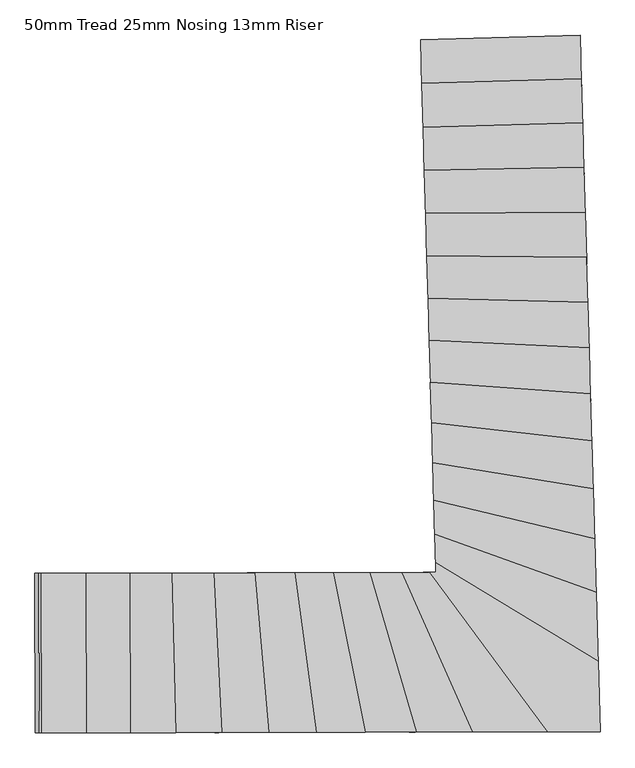
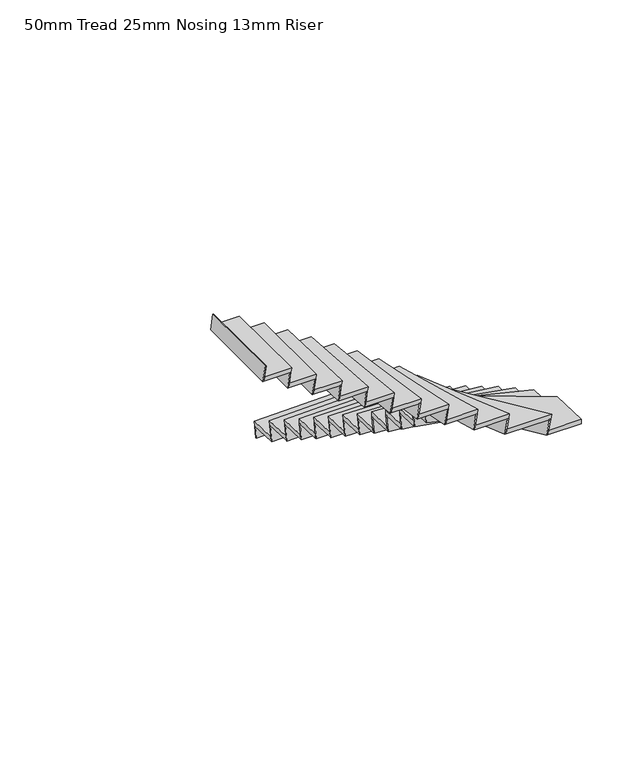
"""IFC4 building model written with IfcOpenShell, lengths in millimetres: stair flight geometry, 50mm Tread 25mm Nosing 13mm Riser."""

from ifc_helpers import new_model, si_unit, origin, place, context, project, spatial, faceted_brep, source, transform, mapped, element, save


def stair_flight_50mm_tread_25mm_nosing_13mm_riser_f5a85d6c(model_context):
    return source(origin(), model_context, "Body", "Brep", [
        faceted_brep([(2321.7147357, 1667.2815701, 869.5652174), (2321.9208524, 1660.0970261, 819.5652174), (3321.5353503, 1688.7748721, 819.5652174), (3321.3292336, 1695.9594161, 869.5652174), (3312.7261016, 1995.8360342, 869.5652174), (2313.1116037, 1967.1581882, 869.5652174), (2313.3177204, 1959.9736442, 819.5652174), (3312.9322183, 1988.6514903, 819.5652174)], [[[0, 1, 2, 3]], [[3, 4, 5, 0]], [[2, 1, 6, 7]], [[4, 3, 2, 7]], [[0, 5, 6, 1]], [[5, 4, 7, 6]]]),
        faceted_brep([(2313.3177204, 1959.9736442, 819.5652174), (2313.8285314, 1942.16847, 695.6521739), (2314.19068, 1929.5451738, 695.6521739), (2313.679869, 1947.350348, 819.5652174), (3312.9322183, 1988.6514903, 819.5652174), (3313.2943668, 1976.028194, 819.5652174), (3313.8051778, 1958.2230198, 695.6521739), (3313.4430292, 1970.8463161, 695.6521739)], [[[0, 1, 2, 3]], [[4, 5, 6, 7]], [[1, 0, 4, 7]], [[2, 1, 7, 6]], [[3, 2, 6, 5]], [[0, 3, 5, 4]]]),
        faceted_brep([(2321.2039248, 1685.0867443, 993.4782609), (2321.9208524, 1660.0970261, 819.5652174), (2322.283001, 1647.4737298, 819.5652174), (2321.5660733, 1672.463448, 993.4782609), (3320.8184226, 1713.7645903, 993.4782609), (3321.1805712, 1701.141294, 993.4782609), (3321.8974988, 1676.1515758, 819.5652174), (3321.5353503, 1688.7748721, 819.5652174)], [[[0, 1, 2, 3]], [[4, 5, 6, 7]], [[1, 0, 4, 7]], [[2, 1, 7, 6]], [[3, 2, 6, 5]], [[0, 3, 5, 4]]]),
        faceted_brep([(3329.2154379, 1421.0725161, 1043.4782609), (3320.6123059, 1720.9491343, 1043.4782609), (2320.9978081, 1692.2712882, 1043.4782609), (2329.6009401, 1392.3946701, 1043.4782609), (3329.4215546, 1413.8879721, 993.4782609), (2329.8070568, 1385.2101261, 993.4782609), (2321.2039248, 1685.0867443, 993.4782609), (3320.8184226, 1713.7645903, 993.4782609)], [[[0, 1, 2, 3]], [[4, 5, 6, 7]], [[1, 0, 4, 7]], [[3, 2, 6, 5]], [[3, 5, 4, 0]], [[2, 1, 7, 6]]]),
        faceted_brep([(2329.0901291, 1410.1998443, 1167.3913043), (2329.8070568, 1385.2101261, 993.4782609), (2330.1692053, 1372.5868298, 993.4782609), (2329.4522777, 1397.576548, 1167.3913043), (3328.704627, 1438.8776903, 1167.3913043), (3329.0667755, 1426.254394, 1167.3913043), (3329.7837032, 1401.2646759, 993.4782609), (3329.4215546, 1413.8879721, 993.4782609)], [[[0, 1, 2, 3]], [[4, 5, 6, 7]], [[1, 0, 4, 7]], [[2, 1, 7, 6]], [[3, 2, 6, 5]], [[0, 3, 5, 4]]]),
        faceted_brep([(3337.2463555, 1141.1413925, 1217.3913043), (3328.4985103, 1446.0622343, 1217.3913043), (2328.8840124, 1417.3843882, 1217.3913043), (2337.3425041, 1122.5494497, 1217.3913043), (3337.4524827, 1133.9564828, 1167.3913043), (2337.5486313, 1115.36454, 1167.3913043), (2329.0901291, 1410.1998443, 1167.3913043), (3328.704627, 1438.8776903, 1167.3913043)], [[[0, 1, 2, 3]], [[4, 5, 6, 7]], [[1, 0, 4, 7]], [[3, 2, 6, 5]], [[3, 5, 4, 0]], [[2, 1, 7, 6]]]),
        faceted_brep([(2336.8316672, 1140.3555302, 1341.3043478), (2337.5486313, 1115.36454, 1167.3913043), (2337.9107983, 1102.7406012, 1167.3913043), (2337.1938342, 1127.7315914, 1341.3043478), (3336.7355186, 1158.947473, 1341.3043478), (3337.0976855, 1146.3235342, 1341.3043478), (3337.8146497, 1121.3325441, 1167.3913043), (3337.4524827, 1133.9564828, 1167.3913043)], [[[0, 1, 2, 3]], [[4, 5, 6, 7]], [[1, 0, 4, 7]], [[2, 1, 7, 6]], [[3, 2, 6, 5]], [[0, 3, 5, 4]]]),
        faceted_brep([(3345.3034332, 860.2984154, 1391.3043478), (3336.5293914, 1166.1323827, 1391.3043478), (2336.62554, 1147.5404399, 1391.3043478), (2345.058109, 853.6090805, 1391.3043478), (3345.5095998, 853.1121335, 1341.3043478), (2345.2642756, 846.4227986, 1341.3043478), (2336.8316672, 1140.3555302, 1341.3043478), (3336.7355186, 1158.947473, 1341.3043478)], [[[0, 1, 2, 3]], [[4, 5, 6, 7]], [[1, 0, 4, 7]], [[3, 2, 6, 5]], [[3, 5, 4, 0]], [[2, 1, 7, 6]]]),
        faceted_brep([(2344.5471745, 871.4185619, 1515.2173913), (2345.2642756, 846.4227986, 1341.3043478), (2345.6265117, 833.7964487, 1341.3043478), (2344.9094107, 858.792212, 1515.2173913), (3344.7924987, 878.1078968, 1515.2173913), (3345.1547348, 865.4815469, 1515.2173913), (3345.8718359, 840.4857836, 1341.3043478), (3345.5095998, 853.1121335, 1341.3043478)], [[[0, 1, 2, 3]], [[4, 5, 6, 7]], [[1, 0, 4, 7]], [[2, 1, 7, 6]], [[3, 2, 6, 5]], [[0, 3, 5, 4]]]),
        faceted_brep([(3353.3944691, 578.2717666, 1565.2173913), (3344.5863321, 885.2941787, 1565.2173913), (2344.3410079, 878.6048439, 1565.2173913), (2352.7400773, 585.841172, 1565.2173913), (3353.6007213, 571.0825008, 1515.2173913), (2352.9463295, 578.6519062, 1515.2173913), (2344.5471745, 871.4185619, 1515.2173913), (3344.7924987, 878.1078968, 1515.2173913)], [[[0, 1, 2, 3]], [[4, 5, 6, 7]], [[1, 0, 4, 7]], [[3, 2, 6, 5]], [[3, 5, 4, 0]], [[2, 1, 7, 6]]]),
        faceted_brep([(2352.2289306, 603.6580482, 1689.1304348), (2352.9463295, 578.6519062, 1515.2173913), (2353.308716, 566.0203136, 1515.2173913), (2352.5913172, 591.0264556, 1689.1304348), (3352.8833224, 596.0886428, 1689.1304348), (3353.245709, 583.4570502, 1689.1304348), (3353.9631079, 558.4509083, 1515.2173913), (3353.6007213, 571.0825008, 1515.2173913)], [[[0, 1, 2, 3]], [[4, 5, 6, 7]], [[1, 0, 4, 7]], [[2, 1, 7, 6]], [[3, 2, 6, 5]], [[0, 3, 5, 4]]]),
        faceted_brep([(3361.5307026, 294.6696799, 1739.1304348), (3352.6770703, 603.2779086, 1739.1304348), (2352.0226784, 610.847314, 1739.1304348), (2360.3773729, 319.6304049, 1739.1304348), (3361.7371159, 287.4748, 1689.1304348), (2360.5837861, 312.4355251, 1689.1304348), (2352.2289306, 603.6580482, 1689.1304348), (3352.8833224, 596.0886428, 1689.1304348)], [[[0, 1, 2, 3]], [[4, 5, 6, 7]], [[1, 0, 4, 7]], [[3, 2, 6, 5]], [[3, 5, 4, 0]], [[2, 1, 7, 6]]]),
        faceted_brep([(2359.865827, 337.461194, 1863.0434783), (2360.5837861, 312.4355251, 1689.1304348), (2360.9464557, 299.7940686, 1689.1304348), (2360.2284966, 324.8197376, 1863.0434783), (3361.0191568, 312.500469, 1863.0434783), (3361.3818263, 299.8590126, 1863.0434783), (3362.0997854, 274.8333436, 1689.1304348), (3361.7371159, 287.4748, 1689.1304348)], [[[0, 1, 2, 3]], [[4, 5, 6, 7]], [[1, 0, 4, 7]], [[2, 1, 7, 6]], [[3, 2, 6, 5]], [[0, 3, 5, 4]]]),
        faceted_brep([(3369.7289475, 8.9060824, 1913.0434783), (3360.8127436, 319.6953488, 1913.0434783), (2359.6594138, 344.6560739, 1913.0434783), (2367.9535387, 55.550418, 1913.0434783), (3369.9356485, 1.701171, 1863.0434783), (2368.1602397, 48.3455066, 1863.0434783), (2359.865827, 337.461194, 1863.0434783), (3361.0191568, 312.500469, 1863.0434783)], [[[0, 1, 2, 3]], [[4, 5, 6, 7]], [[1, 0, 4, 7]], [[3, 2, 6, 5]], [[3, 5, 4, 0]], [[2, 1, 7, 6]]]),
        faceted_brep([(2367.4412796, 73.4060678, 2036.9565217), (2368.1602397, 48.3455066, 1863.0434783), (2368.5234149, 35.6864248, 1863.0434783), (2367.8044549, 60.746986, 2036.9565217), (3369.2166885, 26.7617322, 2036.9565217), (3369.5798637, 14.1026504, 2036.9565217), (3370.2988237, -10.9579108, 1863.0434783), (3369.9356485, 1.701171, 1863.0434783)], [[[0, 1, 2, 3]], [[4, 5, 6, 7]], [[1, 0, 4, 7]], [[2, 1, 7, 6]], [[3, 2, 6, 5]], [[0, 3, 5, 4]]]),
        faceted_brep([(3378.0155364, -279.9368929, 2086.9565217), (3369.0099874, 33.9666436, 2086.9565217), (2367.2345786, 80.6109792, 2086.9565217), (2375.4429017, -205.5039089, 2086.9565217), (3378.2227467, -287.1595576, 2036.9565217), (2375.650112, -212.7265737, 2036.9565217), (2367.4412796, 73.4060678, 2036.9565217), (3369.2166885, 26.7617322, 2036.9565217)], [[[0, 1, 2, 3]], [[4, 5, 6, 7]], [[1, 0, 4, 7]], [[3, 2, 6, 5]], [[3, 5, 4, 0]], [[2, 1, 7, 6]]]),
        faceted_brep([(2374.9293804, -187.6042614, 2210.8695652), (2375.650112, -212.7265737, 2036.9565217), (2376.0141821, -225.4168485, 2036.9565217), (2375.2934505, -200.2945362, 2210.8695652), (3377.5020151, -262.0372454, 2210.8695652), (3377.8660852, -274.7275201, 2210.8695652), (3378.5868168, -299.8498324, 2036.9565217), (3378.2227467, -287.1595576, 2036.9565217)], [[[0, 1, 2, 3]], [[4, 5, 6, 7]], [[1, 0, 4, 7]], [[2, 1, 7, 6]], [[3, 2, 6, 5]], [[0, 3, 5, 4]]]),
        faceted_brep([(3386.4341649, -573.3823325, 2260.8695652), (3377.2948047, -254.8145806, 2260.8695652), (2374.72217, -180.3815967, 2260.8695652), (2382.8030692, -462.0549135, 2260.8695652), (3386.6422935, -580.6370024, 2210.8695652), (2383.0111978, -469.3095834, 2210.8695652), (2374.9293804, -187.6042614, 2210.8695652), (3377.5020151, -262.0372454, 2210.8695652)], [[[0, 1, 2, 3]], [[4, 5, 6, 7]], [[1, 0, 4, 7]], [[3, 2, 6, 5]], [[3, 5, 4, 0]], [[2, 1, 7, 6]]]),
        faceted_brep([(2382.2872724, -444.075949, 2384.7826087), (2383.0111978, -469.3095834, 2210.8695652), (2383.3768811, -482.0560914, 2210.8695652), (2382.6529558, -456.822457, 2384.7826087), (3385.9183681, -555.403368, 2384.7826087), (3386.2840515, -568.1498759, 2384.7826087), (3387.0079768, -593.3835103, 2210.8695652), (3386.6422935, -580.6370024, 2210.8695652)], [[[0, 1, 2, 3]], [[4, 5, 6, 7]], [[1, 0, 4, 7]], [[2, 1, 7, 6]], [[3, 2, 6, 5]], [[0, 3, 5, 4]]]),
        faceted_brep([(3395.0630187, -874.1555248, 2434.7826087), (3385.7102396, -548.1486981, 2434.7826087), (2382.0791439, -436.8212791, 2434.7826087), (2389.9586651, -711.475227, 2434.7826087), (3395.2728781, -881.4705274, 2384.7826087), (2390.1685245, -718.7902296, 2384.7826087), (2382.2872724, -444.075949, 2384.7826087), (3385.9183681, -555.403368, 2384.7826087)], [[[0, 1, 2, 3]], [[4, 5, 6, 7]], [[1, 0, 4, 7]], [[3, 2, 6, 5]], [[3, 5, 4, 0]], [[2, 1, 7, 6]]]),
        faceted_brep([(2389.4385787, -693.3467423, 2558.6956522), (2390.1685245, -718.7902296, 2384.7826087), (2390.537249, -731.6427426, 2384.7826087), (2389.8073032, -706.1992553, 2558.6956522), (3394.5429323, -856.0270401, 2558.6956522), (3394.9116568, -868.8795531, 2558.6956522), (3395.6416026, -894.3230404, 2384.7826087), (3395.2728781, -881.4705274, 2384.7826087)], [[[0, 1, 2, 3]], [[4, 5, 6, 7]], [[1, 0, 4, 7]], [[2, 1, 7, 6]], [[3, 2, 6, 5]], [[0, 3, 5, 4]]]),
        faceted_brep([(3404.0571281, -1187.6603169, 2608.6956522), (3394.3330728, -848.7120375, 2608.6956522), (2389.2287193, -686.0317397, 2608.6956522), (2396.7614696, -948.598407, 2608.6956522), (3404.2705101, -1195.0981067, 2558.6956522), (2396.9748517, -956.0361968, 2558.6956522), (2389.4385787, -693.3467423, 2558.6956522), (3394.5429323, -856.0270401, 2558.6956522)], [[[0, 1, 2, 3]], [[4, 5, 6, 7]], [[1, 0, 4, 7]], [[3, 2, 6, 5]], [[3, 5, 4, 0]], [[2, 1, 7, 6]]]),
        faceted_brep([(2396.2326532, -930.1656235, 2732.6086957), (2396.9748517, -956.0361968, 2558.6956522), (2397.3497655, -969.1044479, 2558.6956522), (2396.607567, -943.2338745, 2732.6086957), (3403.5283117, -1169.2275333, 2732.6086957), (3403.9032255, -1182.2957844, 2732.6086957), (3404.6454239, -1208.1663578, 2558.6956522), (3404.2705101, -1195.0981067, 2558.6956522)], [[[0, 1, 2, 3]], [[4, 5, 6, 7]], [[1, 0, 4, 7]], [[2, 1, 7, 6]], [[3, 2, 6, 5]], [[0, 3, 5, 4]]]),
        faceted_brep([(3413.7732936, -1526.3335896, 2782.6086957), (3403.3149296, -1161.7897435, 2782.6086957), (2396.0192712, -922.7278336, 2782.6086957), (2402.874186, -1161.6674043, 2782.6086957), (3413.9947937, -1534.054347, 2732.6086957), (2403.095686, -1169.3881617, 2732.6086957), (2396.2326532, -930.1656235, 2732.6086957), (3403.5283117, -1169.2275333, 2732.6086957)], [[[0, 1, 2, 3]], [[4, 5, 6, 7]], [[1, 0, 4, 7]], [[3, 2, 6, 5]], [[3, 5, 4, 0]], [[2, 1, 7, 6]]]),
        faceted_brep([(2402.325251, -1142.5333533, 2906.5217391), (2403.095686, -1169.3881617, 2732.6086957), (2403.4848633, -1182.9535889, 2732.6086957), (2402.7144282, -1156.0987805, 2906.5217391), (3413.2243586, -1507.1995386, 2906.5217391), (3413.6135359, -1520.7649658, 2906.5217391), (3414.383971, -1547.6197742, 2732.6086957), (3413.9947937, -1534.054347, 2732.6086957)], [[[0, 1, 2, 3]], [[4, 5, 6, 7]], [[1, 0, 4, 7]], [[2, 1, 7, 6]], [[3, 2, 6, 5]], [[0, 3, 5, 4]]]),
        faceted_brep([(3426.1978229, -1959.4114307, 2956.5217391), (3413.0028586, -1499.4787812, 2956.5217391), (2402.1037509, -1134.8125959, 2956.5217391), (2408.0894679, -1343.4548172, 2956.5217391), (3426.4430823, -1967.9603562, 2906.5217391), (2408.3347272, -1352.0037427, 2906.5217391), (2402.325251, -1142.5333533, 2906.5217391), (3413.2243586, -1507.1995386, 2906.5217391)], [[[0, 1, 2, 3]], [[4, 5, 6, 7]], [[1, 0, 4, 7]], [[3, 2, 6, 5]], [[3, 5, 4, 0]], [[2, 1, 7, 6]]]),
        faceted_brep([(2407.4816513, -1322.2683494, 3080.4347826), (2408.3347272, -1352.0037427, 2906.5217391), (2408.7656496, -1367.0242674, 2906.5217391), (2407.9125737, -1337.2888741, 3080.4347826), (3425.5900064, -1938.2249629, 3080.4347826), (3426.0209288, -1953.2454876, 3080.4347826), (3426.8740047, -1982.9808809, 2906.5217391), (3426.4430823, -1967.9603562, 2906.5217391)], [[[0, 1, 2, 3]], [[4, 5, 6, 7]], [[1, 0, 4, 7]], [[2, 1, 7, 6]], [[3, 2, 6, 5]], [[0, 3, 5, 4]]]),
        faceted_brep([(3075.5893743, -2372.340088, 3130.4347826), (3438.01674, -2371.3796371, 3130.4347826), (3425.3447471, -1929.6760374, 3130.4347826), (2407.236392, -1313.7194239, 3130.4347826), (2408.9679956, -1374.0773756, 3130.4347826), (2337.1103228, -1374.2678021, 3130.4347826), (3066.6658411, -2372.3637358, 3080.4347826), (2328.1867896, -1374.2914499, 3080.4347826), (2408.9679956, -1374.0773756, 3080.4347826), (2407.4816513, -1322.2683494, 3080.4347826), (3425.5900064, -1938.2249629, 3080.4347826), (3438.01674, -2371.3796371, 3080.4347826)], [[[0, 1, 2, 3, 4, 5]], [[6, 7, 8, 9, 10, 11]], [[1, 0, 6, 11]], [[4, 3, 9, 8]], [[5, 7, 6, 0]], [[3, 2, 10, 9]], [[2, 1, 11, 10]], [[5, 4, 8, 7]]]),
        faceted_brep([(2359.225166, -1374.2091966, 3254.3478261), (2328.1867896, -1374.2914499, 3080.4347826), (2312.5080766, -1374.3329993, 3080.4347826), (2343.5464529, -1374.250746, 3254.3478261), (3097.7042175, -2372.2814825, 3254.3478261), (3082.0255045, -2372.3230319, 3254.3478261), (3050.9871281, -2372.4052852, 3080.4347826), (3066.6658411, -2372.3637358, 3080.4347826)], [[[0, 1, 2, 3]], [[4, 5, 6, 7]], [[1, 0, 4, 7]], [[2, 1, 7, 6]], [[3, 2, 6, 5]], [[0, 3, 5, 4]]]),
        faceted_brep([(2609.8575616, -2373.5743008, 3304.3478261), (3106.6277507, -2372.2578347, 3304.3478261), (2368.1486992, -1374.1855488, 3304.3478261), (2167.530501, -1374.7171972, 3304.3478261), (2602.0060647, -2373.5951077, 3254.3478261), (2159.6790041, -1374.7380041, 3254.3478261), (2359.225166, -1374.2091966, 3254.3478261), (3097.7042175, -2372.2814825, 3254.3478261)], [[[0, 1, 2, 3]], [[4, 5, 6, 7]], [[1, 0, 4, 7]], [[3, 2, 6, 5]], [[3, 5, 4, 0]], [[2, 1, 7, 6]]]),
        faceted_brep([(2186.9885586, -1374.6656324, 3428.2608696), (2159.6790041, -1374.7380041, 3254.3478261), (2145.8838666, -1374.7745619, 3254.3478261), (2173.1934212, -1374.7021902, 3428.2608696), (2629.3156193, -2373.522736, 3428.2608696), (2615.5204818, -2373.5592938, 3428.2608696), (2588.2109272, -2373.6316655, 3254.3478261), (2602.0060647, -2373.5951077, 3254.3478261)], [[[0, 1, 2, 3]], [[4, 5, 6, 7]], [[1, 0, 4, 7]], [[2, 1, 7, 6]], [[3, 2, 6, 5]], [[0, 3, 5, 4]]]),
        faceted_brep([(2260.9356063, -2374.4989617, 3478.2608696), (2637.1671162, -2373.5019291, 3478.2608696), (2194.8400556, -1374.6448255, 3478.2608696), (1968.9950491, -1375.2433262, 3478.2608696), (2253.4534305, -2374.5187898, 3428.2608696), (1961.5128732, -1375.2631543, 3428.2608696), (2186.9885586, -1374.6656324, 3428.2608696), (2629.3156193, -2373.522736, 3428.2608696)], [[[0, 1, 2, 3]], [[4, 5, 6, 7]], [[1, 0, 4, 7]], [[3, 2, 6, 5]], [[3, 5, 4, 0]], [[2, 1, 7, 6]]]),
        faceted_brep([(1987.5378327, -1375.1941869, 3602.173913), (1961.5128732, -1375.2631543, 3428.2608696), (1948.3666356, -1375.2979925, 3428.2608696), (1974.3915951, -1375.2290251, 3602.173913), (2279.4783899, -2374.4498223, 3602.173913), (2266.3321523, -2374.4846605, 3602.173913), (2240.3071928, -2374.553628, 3428.2608696), (2253.4534305, -2374.5187898, 3428.2608696)], [[[0, 1, 2, 3]], [[4, 5, 6, 7]], [[1, 0, 4, 7]], [[2, 1, 7, 6]], [[3, 2, 6, 5]], [[0, 3, 5, 4]]]),
        faceted_brep([(1939.6520151, -2375.3503794, 3652.173913), (2286.9605658, -2374.4299942, 3652.173913), (1995.0200086, -1375.1743587, 3652.173913), (1741.3830236, -1375.8465096, 3652.173913), (1932.3283168, -2375.3697876, 3602.173913), (1734.0593253, -1375.8659177, 3602.173913), (1987.5378327, -1375.1941869, 3602.173913), (2279.4783899, -2374.4498223, 3602.173913)], [[[0, 1, 2, 3]], [[4, 5, 6, 7]], [[1, 0, 4, 7]], [[3, 2, 6, 5]], [[3, 5, 4, 0]], [[2, 1, 7, 6]]]),
        faceted_brep([(1759.5330587, -1375.7984111, 3776.0869565), (1734.0593253, -1375.8659177, 3602.173913), (1721.1915338, -1375.900018, 3602.173913), (1746.6652672, -1375.8325114, 3776.0869565), (1957.8020502, -2375.3022809, 3776.0869565), (1944.9342587, -2375.3363812, 3776.0869565), (1919.4605252, -2375.4038879, 3602.173913), (1932.3283168, -2375.3697876, 3602.173913)], [[[0, 1, 2, 3]], [[4, 5, 6, 7]], [[1, 0, 4, 7]], [[2, 1, 7, 6]], [[3, 2, 6, 5]], [[0, 3, 5, 4]]]),
        faceted_brep([(1632.9356634, -2376.1631933, 3826.0869565), (1965.1257485, -2375.2828727, 3826.0869565), (1766.8567571, -1375.7790029, 3826.0869565), (1498.6174196, -1376.4898507, 3826.0869565), (1625.6861563, -2376.1824048, 3776.0869565), (1491.3679125, -1376.5090623, 3776.0869565), (1759.5330587, -1375.7984111, 3776.0869565), (1957.8020502, -2375.3022809, 3776.0869565)], [[[0, 1, 2, 3]], [[4, 5, 6, 7]], [[1, 0, 4, 7]], [[3, 2, 6, 5]], [[3, 5, 4, 0]], [[2, 1, 7, 6]]]),
        faceted_brep([(1516.5835894, -1376.4422394, 3950.0), (1491.3679125, -1376.5090623, 3776.0869565), (1478.6304755, -1376.5428171, 3776.0869565), (1503.8461525, -1376.4759943, 3950.0), (1650.9018332, -2376.115582, 3950.0), (1638.1643962, -2376.1493369, 3950.0), (1612.9487193, -2376.2161597, 3776.0869565), (1625.6861563, -2376.1824048, 3776.0869565)], [[[0, 1, 2, 3]], [[4, 5, 6, 7]], [[1, 0, 4, 7]], [[2, 1, 7, 6]], [[3, 2, 6, 5]], [[0, 3, 5, 4]]]),
        faceted_brep([(1334.8426475, -2376.9531549, 4000.0), (1658.1513403, -2376.0963705, 4000.0), (1523.8330965, -1376.4230279, 4000.0), (1246.96263, -1377.1567486, 4000.0), (1327.6291158, -2376.9722711, 3950.0), (1239.7490983, -1377.1758648, 3950.0), (1516.5835894, -1376.4422394, 3950.0), (1650.9018332, -2376.115582, 3950.0)], [[[0, 1, 2, 3]], [[4, 5, 6, 7]], [[1, 0, 4, 7]], [[3, 2, 6, 5]], [[3, 5, 4, 0]], [[2, 1, 7, 6]]]),
        faceted_brep([(1264.8396435, -1377.1093736, 4123.9130435), (1239.7490983, -1377.1758648, 3950.0), (1227.0748702, -1377.2094522, 3950.0), (1252.1654155, -1377.142961, 4123.9130435), (1352.719661, -2376.9057799, 4123.9130435), (1340.045433, -2376.9393672, 4123.9130435), (1314.9548878, -2377.0058584, 3950.0), (1327.6291158, -2376.9722711, 3950.0)], [[[0, 1, 2, 3]], [[4, 5, 6, 7]], [[1, 0, 4, 7]], [[2, 1, 7, 6]], [[3, 2, 6, 5]], [[0, 3, 5, 4]]]),
        faceted_brep([(1042.2765878, -2377.7284697, 4173.9130435), (1359.9331928, -2376.8866636, 4173.9130435), (1272.0531753, -1377.0902574, 4173.9130435), (989.6494865, -1377.8386415, 4173.9130435), (1035.080143, -2377.7475407, 4123.9130435), (982.4530417, -1377.8577124, 4123.9130435), (1264.8396435, -1377.1093736, 4123.9130435), (1352.719661, -2376.9057799, 4123.9130435)], [[[0, 1, 2, 3]], [[4, 5, 6, 7]], [[1, 0, 4, 7]], [[3, 2, 6, 5]], [[3, 5, 4, 0]], [[2, 1, 7, 6]]]),
        faceted_brep([(1007.4841542, -1377.7913787, 4297.826087), (982.4530417, -1377.8577124, 4123.9130435), (969.8088355, -1377.8912202, 4123.9130435), (994.839948, -1377.8248865, 4297.826087), (1060.1112555, -2377.6812069, 4297.826087), (1047.4670493, -2377.7147147, 4297.826087), (1022.4359369, -2377.7810484, 4123.9130435), (1035.080143, -2377.7475407, 4123.9130435)], [[[0, 1, 2, 3]], [[4, 5, 6, 7]], [[1, 0, 4, 7]], [[2, 1, 7, 6]], [[3, 2, 6, 5]], [[0, 3, 5, 4]]]),
        faceted_brep([(753.4653173, -2378.4938342, 4347.826087), (1067.3077003, -2377.662136, 4347.826087), (1014.680599, -1377.7723078, 4347.826087), (728.5126559, -1378.5306673, 4347.826087), (746.2760553, -2378.5128861, 4297.826087), (721.3233939, -1378.5497192, 4297.826087), (1007.4841542, -1377.7913787, 4297.826087), (1060.1112555, -2377.6812069, 4297.826087)], [[[0, 1, 2, 3]], [[4, 5, 6, 7]], [[1, 0, 4, 7]], [[3, 2, 6, 5]], [[3, 5, 4, 0]], [[2, 1, 7, 6]]]),
        faceted_brep([(746.3295226, -1378.4834517, 4471.7391304), (721.3233939, -1378.5497192, 4297.826087), (708.6918081, -1378.5831935, 4297.826087), (733.6979368, -1378.516926, 4471.7391304), (771.282184, -2378.4466186, 4471.7391304), (758.6505982, -2378.4800929, 4471.7391304), (733.6444695, -2378.5463604, 4297.826087), (746.2760553, -2378.5128861, 4297.826087)], [[[0, 1, 2, 3]], [[4, 5, 6, 7]], [[1, 0, 4, 7]], [[2, 1, 7, 6]], [[3, 2, 6, 5]], [[0, 3, 5, 4]]]),
        faceted_brep([(467.3212235, -2379.2521305, 4521.7391304), (778.471446, -2378.4275667, 4521.7391304), (753.5187846, -1378.4643998, 4521.7391304), (464.6711139, -1379.2298607, 4521.7391304), (460.1337488, -2379.2711777, 4471.7391304), (457.4836392, -1379.2489079, 4471.7391304), (746.3295226, -1378.4834517, 4471.7391304), (771.282184, -2378.4466186, 4471.7391304)], [[[0, 1, 2, 3]], [[4, 5, 6, 7]], [[1, 0, 4, 7]], [[3, 2, 6, 5]], [[3, 5, 4, 0]], [[2, 1, 7, 6]]]),
        faceted_brep([(482.4835514, -1379.1826569, 4645.6521739), (457.4836392, -1379.2489079, 4471.7391304), (444.8551935, -1379.2823739, 4471.7391304), (469.8551057, -1379.2161229, 4645.6521739), (485.133661, -2379.2049266, 4645.6521739), (472.5052153, -2379.2383927, 4645.6521739), (447.5053031, -2379.3046437, 4471.7391304), (460.1337488, -2379.2711777, 4471.7391304)], [[[0, 1, 2, 3]], [[4, 5, 6, 7]], [[1, 0, 4, 7]], [[2, 1, 7, 6]], [[3, 2, 6, 5]], [[0, 3, 5, 4]]]),
        faceted_brep([(192.3221891, -2379.9808919, 4695.6521739), (492.3211357, -2379.1858795, 4695.6521739), (489.6710261, -1379.1636097, 4695.6521739), (189.6720795, -1379.9586221, 4695.6521739), (185.1347144, -2379.999939, 4645.6521739), (182.4846048, -1379.9776692, 4645.6521739), (482.4835514, -1379.1826569, 4645.6521739), (485.133661, -2379.2049266, 4645.6521739)], [[[0, 1, 2, 3]], [[4, 5, 6, 7]], [[1, 0, 4, 7]], [[3, 2, 6, 5]], [[3, 5, 4, 0]], [[2, 1, 7, 6]]]),
        faceted_brep([(207.484517, -1379.9114182, 4819.5652174), (182.4846048, -1379.9776692, 4645.6521739), (169.8561591, -1380.0111353, 4645.6521739), (194.8560713, -1379.9448842, 4819.5652174), (210.1346266, -2379.933688, 4819.5652174), (197.5061809, -2379.967154, 4819.5652174), (172.5062687, -2380.0334051, 4645.6521739), (185.1347144, -2379.999939, 4645.6521739)], [[[0, 1, 2, 3]], [[4, 5, 6, 7]], [[1, 0, 4, 7]], [[2, 1, 7, 6]], [[3, 2, 6, 5]], [[0, 3, 5, 4]]]),
        faceted_brep([(-67.5145174, -1380.6401796, 4993.4782609), (-92.5144296, -1380.7064306, 4819.5652174), (-105.1428753, -1380.7398966, 4819.5652174), (-80.142963, -1380.6736456, 4993.4782609), (-64.8644078, -2380.6624494, 4993.4782609), (-77.4928534, -2380.6959154, 4993.4782609), (-102.4927657, -2380.7621664, 4819.5652174), (-89.86432, -2380.7287004, 4819.5652174)], [[[0, 1, 2, 3]], [[4, 5, 6, 7]], [[1, 0, 4, 7]], [[2, 1, 7, 6]], [[3, 2, 6, 5]], [[0, 3, 5, 4]]]),
        faceted_brep([(-82.6768452, -2380.7096532, 4869.5652174), (217.3221014, -2379.9146408, 4869.5652174), (214.6719918, -1379.892371, 4869.5652174), (-85.3269548, -1380.6873834, 4869.5652174), (-89.86432, -2380.7287004, 4819.5652174), (-92.5144296, -1380.7064306, 4819.5652174), (207.484517, -1379.9114182, 4819.5652174), (210.1346266, -2379.933688, 4819.5652174)], [[[0, 1, 2, 3]], [[4, 5, 6, 7]], [[1, 0, 4, 7]], [[3, 2, 6, 5]], [[3, 5, 4, 0]], [[2, 1, 7, 6]]]),
    ])


if __name__ == "__main__":
    model = new_model("IFC4")
    model_context = context("Model", 3, world=origin())
    ifc_project = project(units=[si_unit("LENGTHUNIT", "METRE", prefix="MILLI")], contexts=[model_context])
    site = spatial("IfcSite", under=ifc_project)
    building = spatial("IfcBuilding", under=site)
    placement = place(None, origin())
    stair_flight_50mm_tread_25mm_nosing_13mm_riser_shape = stair_flight_50mm_tread_25mm_nosing_13mm_riser_f5a85d6c(model_context)
    element("IfcStairFlight", 1, ObjectType="50mm Tread 25mm Nosing 13mm Riser", at=placement, inside=building, context=model_context, shape_type="MappedRepresentation", body=[
        mapped(stair_flight_50mm_tread_25mm_nosing_13mm_riser_shape, transform((0.0, 0.0, 0.0), x_axis=(1.0, 0.0, 0.0), y_axis=(0.0, 1.0, 0.0), z_axis=(0.0, 0.0, 1.0))),
    ])
    save(model, "model.ifc")
